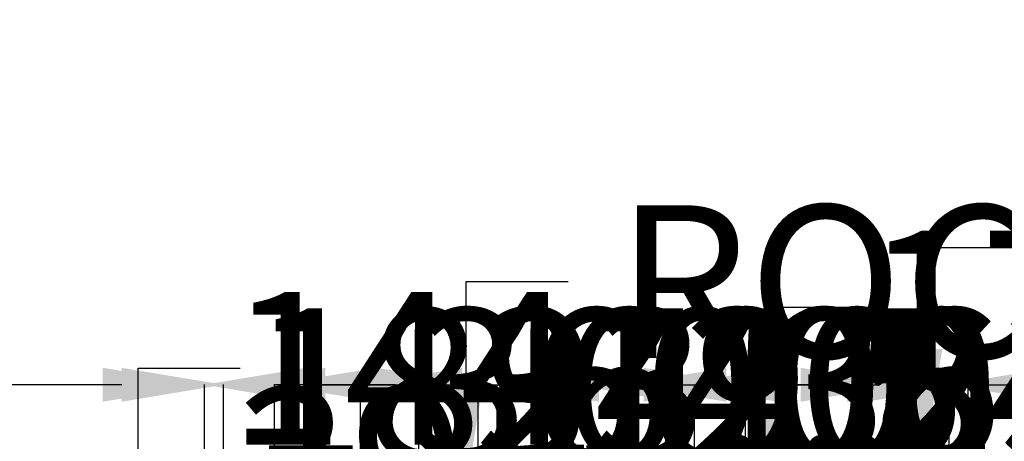
# Model space of a CAD drawing. Units: inches. Extents: x -307 to 2141, y -58 to 895.
# Tile 25 of 28: x 469 to 933, y 696 to 895. Entities that reach past the tile are written whole.
import ezdxf

# ---------------------------------------------------------------- set-up
doc = ezdxf.new("R2010")
doc.units = ezdxf.units.IN
doc.header["$MEASUREMENT"] = 0
doc.layers.add('A-ANNO-DIMS', color=2, linetype='Continuous', lineweight=18)
doc.styles.get("Standard").update_dxf_attribs({"font": 'arial.ttf'})
doc.dimstyles.get("Standard").update_dxf_attribs({"dimtxt": 72, "dimasz": 48, "dimexe": 0.18, "dimexo": 0.0625, "dimgap": 0.09, "dimtad": 0, "dimtih": 1, "dimtoh": 1, "dimdec": 0, "dimrnd": 48, "dimzin": 0, "dimdsep": 46, "dimlunit": 3, "dimtxsty": 'Standard', "dimcen": 0.09, "dimadec": 0, "dimazin": 0, "dimtfac": 1, "dimtdec": 0, "dimtofl": 0, "dimtmove": 0, "dimatfit": 3, "dimfxl": 1, "dimtolj": 1, "dimtzin": 0, "dimarcsym": 0})

# ---------------------------------------------------------------- blocks, each defined once
blk = doc.blocks.new('*D26')
at = {"layer": 'A-ANNO-DIMS', "color": 0, "lineweight": -2, "transparency": 16777216}
for p, q in [((565.34, 584.2), (565.34, 572.08)), ((645.34, 584.2), (645.34, 572.08)), ((517.34, 572.26), (469.34, 572.26)), ((693.34, 572.26), (741.34, 572.26))]:
    blk.add_line(p, q, dxfattribs=at)
at = {"layer": 'A-ANNO-DIMS', "color": 0, "transparency": 16777216}
for points in [[(517.34, 580.26), (517.34, 564.26), (565.34, 572.26)], [(693.34, 580.26), (693.34, 564.26), (645.34, 572.26)]]:
    blk.add_solid(points, dxfattribs=at)
at = {"layer": 'Defpoints', "color": 0, "transparency": 16777216}
for p in [(565.34, 584.26), (645.34, 584.26), (565.34, 572.26)]:
    blk.add_point(p, dxfattribs=at)
at = {"layer": 'A-ANNO-DIMS', "color": 0, "transparency": 16777216, "insert": (178.23, 572.26), "char_height": 72, "attachment_point": 5}
blk.add_mtext('\\A1;BED 80 TYP.', dxfattribs=at)
blk = doc.blocks.new('*D27')
at = {"layer": 'A-ANNO-DIMS', "color": 0, "lineweight": -2, "transparency": 16777216}
for p, q in [((657.34, 692.26), (657.34, 740.26)), ((645.4, 644.26), (657.52, 644.26)), ((645.4, 584.26), (657.52, 584.26)), ((657.34, 536.26), (657.34, 488.26)), ((657.34, 488.26), (609.34, 488.26))]:
    blk.add_line(p, q, dxfattribs=at)
at = {"layer": 'A-ANNO-DIMS', "color": 0, "transparency": 16777216}
for points in [[(649.34, 692.26), (665.34, 692.26), (657.34, 644.26)], [(649.34, 536.26), (665.34, 536.26), (657.34, 584.26)]]:
    blk.add_solid(points, dxfattribs=at)
at = {"layer": 'Defpoints', "color": 0, "transparency": 16777216}
for p in [(645.34, 644.26), (645.34, 584.26), (657.34, 584.26)]:
    blk.add_point(p, dxfattribs=at)
at = {"layer": 'A-ANNO-DIMS', "color": 0, "transparency": 16777216, "insert": (433.81, 488.26), "char_height": 72, "attachment_point": 5}
blk.add_mtext('\\A1;60 TYP.', dxfattribs=at)
blk = doc.blocks.new('*D30')
at = {"layer": 'A-ANNO-DIMS', "color": 0, "lineweight": -2, "transparency": 16777216}
for p, q in [((570.74, 532.83), (570.74, 580.83)), ((570.74, 580.83), (618.74, 580.83)), ((565.4, 484.83), (570.92, 484.83)), ((565.4, 448.83), (570.92, 448.83)), ((570.74, 400.83), (570.74, 352.83))]:
    blk.add_line(p, q, dxfattribs=at)
at = {"layer": 'A-ANNO-DIMS', "color": 0, "transparency": 16777216}
for points in [[(562.74, 532.83), (578.74, 532.83), (570.74, 484.83)], [(562.74, 400.83), (578.74, 400.83), (570.74, 448.83)]]:
    blk.add_solid(points, dxfattribs=at)
at = {"layer": 'Defpoints', "color": 0, "transparency": 16777216}
for p in [(565.34, 484.83), (570.74, 484.83), (565.34, 448.83)]:
    blk.add_point(p, dxfattribs=at)
at = {"layer": 'A-ANNO-DIMS', "color": 0, "transparency": 16777216, "insert": (1030.17, 580.83), "char_height": 72, "attachment_point": 5}
blk.add_mtext('\\A1;WINDOW 36 TYP.', dxfattribs=at)
blk = doc.blocks.new('*D32')
at = {"layer": 'A-ANNO-DIMS', "color": 0, "lineweight": -2, "transparency": 16777216}
for p, q in [((813.29, 682.28), (813.29, 671.36)), ((885.29, 682.28), (885.29, 671.36)), ((765.29, 671.54), (717.29, 671.54)), ((933.29, 671.54), (981.29, 671.54))]:
    blk.add_line(p, q, dxfattribs=at)
at = {"layer": 'A-ANNO-DIMS', "color": 0, "transparency": 16777216}
for points in [[(765.29, 679.54), (765.29, 663.54), (813.29, 671.54)], [(933.29, 679.54), (933.29, 663.54), (885.29, 671.54)]]:
    blk.add_solid(points, dxfattribs=at)
at = {"layer": 'Defpoints', "color": 0, "transparency": 16777216}
for p in [(813.29, 682.34), (885.29, 682.34), (885.29, 671.54)]:
    blk.add_point(p, dxfattribs=at)
at = {"layer": 'A-ANNO-DIMS', "color": 0, "transparency": 16777216, "insert": (1392.73, 671.54), "char_height": 72, "attachment_point": 5}
blk.add_mtext('\\A1;WINDOW 72 TYP.', dxfattribs=at)
blk = doc.blocks.new('*D33')
at = {"layer": 'A-ANNO-DIMS', "color": 0, "lineweight": -2, "transparency": 16777216}
for p, q in [((896.09, 739.34), (896.09, 787.34)), ((896.09, 787.34), (944.09, 787.34)), ((885.36, 691.34), (896.27, 691.34)), ((885.36, 682.34), (896.27, 682.34)), ((896.09, 634.34), (896.09, 586.34))]:
    blk.add_line(p, q, dxfattribs=at)
at = {"layer": 'A-ANNO-DIMS', "color": 0, "transparency": 16777216}
for points in [[(888.09, 739.34), (904.09, 739.34), (896.09, 691.34)], [(888.09, 634.34), (904.09, 634.34), (896.09, 682.34)]]:
    blk.add_solid(points, dxfattribs=at)
at = {"layer": 'Defpoints', "color": 0, "transparency": 16777216}
for p in [(885.29, 691.34), (896.09, 691.34), (885.29, 682.34)]:
    blk.add_point(p, dxfattribs=at)
at = {"layer": 'A-ANNO-DIMS', "color": 0, "transparency": 16777216, "insert": (1091.45, 787.34), "char_height": 72, "attachment_point": 5}
blk.add_mtext('\\A1;9 TYP.', dxfattribs=at)
blk = doc.blocks.new('*D34')
at = {"layer": 'A-ANNO-DIMS', "color": 0, "lineweight": -2, "transparency": 16777216}
for p, q in [((927.14, 490.97), (927.14, 538.97)), ((927.14, 538.97), (975.14, 538.97)), ((916.4, 442.97), (927.32, 442.97)), ((916.4, 370.95), (927.32, 370.95)), ((927.14, 322.95), (927.14, 274.95))]:
    blk.add_line(p, q, dxfattribs=at)
at = {"layer": 'A-ANNO-DIMS', "color": 0, "transparency": 16777216}
for points in [[(919.14, 490.97), (935.14, 490.97), (927.14, 442.97)], [(919.14, 322.95), (935.14, 322.95), (927.14, 370.95)]]:
    blk.add_solid(points, dxfattribs=at)
at = {"layer": 'Defpoints', "color": 0, "transparency": 16777216}
for p in [(916.34, 442.97), (927.14, 442.97), (916.34, 370.95)]:
    blk.add_point(p, dxfattribs=at)
at = {"layer": 'A-ANNO-DIMS', "color": 0, "transparency": 16777216, "insert": (1584.53, 538.97), "char_height": 72, "attachment_point": 5}
blk.add_mtext('\\A1;PAIRED WINDOW 72 TYP.', dxfattribs=at)
blk = doc.blocks.new('*D46')
at = {"layer": 'A-ANNO-DIMS', "color": 0, "lineweight": -2, "transparency": 16777216}
for p, q in [((801.41, 645.78), (801.41, 642.52)), ((822.41, 645.78), (822.41, 642.52)), ((753.41, 642.7), (705.41, 642.7)), ((870.41, 642.7), (918.41, 642.7))]:
    blk.add_line(p, q, dxfattribs=at)
at = {"layer": 'A-ANNO-DIMS', "color": 0, "transparency": 16777216}
for points in [[(753.41, 650.7), (753.41, 634.7), (801.41, 642.7)], [(870.41, 650.7), (870.41, 634.7), (822.41, 642.7)]]:
    blk.add_solid(points, dxfattribs=at)
at = {"layer": 'Defpoints', "color": 0, "transparency": 16777216}
for p in [(801.41, 645.85), (822.41, 645.85), (822.41, 642.7)]:
    blk.add_point(p, dxfattribs=at)
at = {"layer": 'A-ANNO-DIMS', "color": 0, "transparency": 16777216, "insert": (1282.7, 642.7), "char_height": 72, "attachment_point": 5}
blk.add_mtext('\\A1;DESK CHAIR 21', dxfattribs=at)
blk = doc.blocks.new('*D47')
at = {"layer": 'A-ANNO-DIMS', "color": 0, "lineweight": -2, "transparency": 16777216}
for p, q in [((825.56, 711.18), (825.56, 759.18)), ((825.56, 759.18), (873.56, 759.18)), ((822.48, 663.18), (825.74, 663.18)), ((822.48, 645.85), (825.74, 645.85)), ((825.56, 597.85), (825.56, 549.85))]:
    blk.add_line(p, q, dxfattribs=at)
at = {"layer": 'A-ANNO-DIMS', "color": 0, "transparency": 16777216}
for points in [[(817.56, 711.18), (833.56, 711.18), (825.56, 663.18)], [(817.56, 597.85), (833.56, 597.85), (825.56, 645.85)]]:
    blk.add_solid(points, dxfattribs=at)
at = {"layer": 'Defpoints', "color": 0, "transparency": 16777216}
for p in [(822.41, 663.18), (825.56, 663.18), (822.41, 645.85)]:
    blk.add_point(p, dxfattribs=at)
at = {"layer": 'A-ANNO-DIMS', "color": 0, "transparency": 16777216, "insert": (921.83, 759.18), "char_height": 72, "attachment_point": 5}
blk.add_mtext('\\A1;17', dxfattribs=at)
blk = doc.blocks.new('*D56')
at = {"layer": 'A-ANNO-DIMS', "color": 0, "lineweight": -2, "transparency": 16777216}
for p, q in [((679.73, 723.21), (679.73, 771.21)), ((679.73, 771.21), (727.73, 771.21)), ((675.74, 675.21), (679.91, 675.21)), ((675.74, 648.21), (679.91, 648.21)), ((679.73, 600.21), (679.73, 552.21))]:
    blk.add_line(p, q, dxfattribs=at)
at = {"layer": 'A-ANNO-DIMS', "color": 0, "transparency": 16777216}
for points in [[(671.73, 723.21), (687.73, 723.21), (679.73, 675.21)], [(671.73, 600.21), (687.73, 600.21), (679.73, 648.21)]]:
    blk.add_solid(points, dxfattribs=at)
at = {"layer": 'Defpoints', "color": 0, "transparency": 16777216}
for p in [(675.68, 675.21), (679.73, 675.21), (675.68, 648.21)]:
    blk.add_point(p, dxfattribs=at)
at = {"layer": 'A-ANNO-DIMS', "color": 0, "transparency": 16777216, "insert": (1006.66, 771.21), "char_height": 72, "attachment_point": 5}
blk.add_mtext('\\A1;ROCKER 27', dxfattribs=at)
blk = doc.blocks.new('*D62')
at = {"layer": 'A-ANNO-DIMS', "color": 0, "lineweight": -2, "transparency": 16777216}
for p, q in [((556.34, 691.4), (556.34, 722.72)), ((604.34, 722.54), (656.85, 722.54)), ((868.34, 722.54), (815.82, 722.54)), ((916.34, 490.97), (916.34, 722.72))]:
    blk.add_line(p, q, dxfattribs=at)
at = {"layer": 'A-ANNO-DIMS', "color": 0, "transparency": 16777216}
for points in [[(604.34, 730.54), (604.34, 714.54), (556.34, 722.54)], [(868.34, 730.54), (868.34, 714.54), (916.34, 722.54)]]:
    blk.add_solid(points, dxfattribs=at)
at = {"layer": 'Defpoints', "color": 0, "transparency": 16777216}
for p in [(916.34, 722.54), (556.34, 691.34), (916.34, 490.9)]:
    blk.add_point(p, dxfattribs=at)
at = {"layer": 'A-ANNO-DIMS', "color": 0, "transparency": 16777216, "insert": (736.34, 722.54), "char_height": 72, "attachment_point": 5}
blk.add_mtext('\\A1;360', dxfattribs=at)
blk = doc.blocks.new('*D69')
at = {"layer": 'A-ANNO-DIMS', "color": 0, "lineweight": -2, "transparency": 16777216}
for p, q in [((525.13, 682.34), (525.13, 730.34)), ((525.13, 730.34), (573.13, 730.34)), ((565.27, 682.34), (524.95, 682.34)), ((525.13, 586.34), (525.13, 634.34)), ((565.27, 538.34), (524.95, 538.34))]:
    blk.add_line(p, q, dxfattribs=at)
at = {"layer": 'A-ANNO-DIMS', "color": 0, "transparency": 16777216}
for points in [[(517.13, 634.34), (533.13, 634.34), (525.13, 682.34)], [(517.13, 586.34), (533.13, 586.34), (525.13, 538.34)]]:
    blk.add_solid(points, dxfattribs=at)
at = {"layer": 'Defpoints', "color": 0, "transparency": 16777216}
for p in [(525.13, 682.34), (565.34, 682.34), (565.34, 538.34)]:
    blk.add_point(p, dxfattribs=at)
at = {"layer": 'A-ANNO-DIMS', "color": 0, "transparency": 16777216, "insert": (649.22, 730.34), "char_height": 72, "attachment_point": 5}
blk.add_mtext('\\A1;144', dxfattribs=at)
blk = doc.blocks.new('*D75')
at = {"layer": 'A-ANNO-DIMS', "color": 0, "lineweight": -2, "transparency": 16777216}
for p, q in [((565.34, 682.4), (565.34, 722.72)), ((613.34, 722.54), (637.34, 722.54)), ((685.34, 682.4), (685.34, 722.72)), ((685.34, 722.54), (733.34, 722.54))]:
    blk.add_line(p, q, dxfattribs=at)
at = {"layer": 'A-ANNO-DIMS', "color": 0, "transparency": 16777216}
for points in [[(613.34, 730.54), (613.34, 714.54), (565.34, 722.54)], [(637.34, 730.54), (637.34, 714.54), (685.34, 722.54)]]:
    blk.add_solid(points, dxfattribs=at)
at = {"layer": 'Defpoints', "color": 0, "transparency": 16777216}
for p in [(685.34, 722.54), (565.34, 682.34), (685.34, 682.34)]:
    blk.add_point(p, dxfattribs=at)
at = {"layer": 'A-ANNO-DIMS', "color": 0, "transparency": 16777216, "insert": (809.45, 722.54), "char_height": 72, "attachment_point": 5}
blk.add_mtext('\\A1;120', dxfattribs=at)
blk = doc.blocks.new('*D76')
at = {"layer": 'A-ANNO-DIMS', "color": 0, "lineweight": -2, "transparency": 16777216}
for p, q in [((646.34, 722.54), (598.34, 722.54)), ((694.34, 682.4), (694.34, 722.72)), ((778.34, 682.4), (778.34, 722.72)), ((826.34, 722.54), (874.34, 722.54))]:
    blk.add_line(p, q, dxfattribs=at)
at = {"layer": 'A-ANNO-DIMS', "color": 0, "transparency": 16777216}
for points in [[(646.34, 730.54), (646.34, 714.54), (694.34, 722.54)], [(826.34, 730.54), (826.34, 714.54), (778.34, 722.54)]]:
    blk.add_solid(points, dxfattribs=at)
at = {"layer": 'Defpoints', "color": 0, "transparency": 16777216}
for p in [(778.34, 722.54), (694.34, 682.34), (778.34, 682.34)]:
    blk.add_point(p, dxfattribs=at)
at = {"layer": 'A-ANNO-DIMS', "color": 0, "transparency": 16777216, "insert": (925.9, 722.54), "char_height": 72, "attachment_point": 5}
blk.add_mtext('\\A1;84', dxfattribs=at)
blk = doc.blocks.new('*D77')
at = {"layer": 'A-ANNO-DIMS', "color": 0, "lineweight": -2, "transparency": 16777216}
for p, q in [((787.34, 682.4), (787.34, 722.72)), ((835.34, 722.54), (859.34, 722.54)), ((907.34, 682.4), (907.34, 722.72)), ((907.34, 722.54), (955.34, 722.54))]:
    blk.add_line(p, q, dxfattribs=at)
at = {"layer": 'A-ANNO-DIMS', "color": 0, "transparency": 16777216}
for points in [[(835.34, 730.54), (835.34, 714.54), (787.34, 722.54)], [(859.34, 730.54), (859.34, 714.54), (907.34, 722.54)]]:
    blk.add_solid(points, dxfattribs=at)
at = {"layer": 'Defpoints', "color": 0, "transparency": 16777216}
for p in [(907.34, 722.54), (787.34, 682.34), (907.34, 682.34)]:
    blk.add_point(p, dxfattribs=at)
at = {"layer": 'A-ANNO-DIMS', "color": 0, "transparency": 16777216, "insert": (1031.45, 722.54), "char_height": 72, "attachment_point": 5}
blk.add_mtext('\\A1;120', dxfattribs=at)
blk = doc.blocks.new('*D78')
at = {"layer": 'A-ANNO-DIMS', "color": 0, "lineweight": -2, "transparency": 16777216}
for p, q in [((947.53984, 730.340828), (947.53984, 778.340828)), ((778.39834, 682.340828), (947.71984, 682.340828)), ((730.39834, 598.340828), (947.71984, 598.340828)), ((947.53984, 550.340828), (947.53984, 502.340828))]:
    blk.add_line(p, q, dxfattribs=at)
at = {"layer": 'A-ANNO-DIMS', "color": 0, "transparency": 16777216}
for points in [[(939.53984, 730.340828), (955.53984, 730.340828), (947.53984, 682.340828)], [(939.53984, 550.340828), (955.53984, 550.340828), (947.53984, 598.340828)]]:
    blk.add_solid(points, dxfattribs=at)
at = {"layer": 'Defpoints', "color": 0, "transparency": 16777216}
for p in [(778.33584, 682.340828), (947.53984, 682.340828), (730.33584, 598.340828)]:
    blk.add_point(p, dxfattribs=at)
at = {"layer": 'A-ANNO-DIMS', "color": 0, "transparency": 16777216, "insert": (947.53984, 640.340828), "char_height": 72, "attachment_point": 5}
blk.add_mtext('\\A1;84', dxfattribs=at)
blk = doc.blocks.new('*D79')
at = {"layer": 'A-ANNO-DIMS', "color": 0, "lineweight": -2, "transparency": 16777216}
for p, q in [((947.54, 682.34), (947.54, 730.34)), ((947.54, 730.34), (995.54, 730.34)), ((907.4, 682.34), (947.72, 682.34)), ((947.54, 598.34), (947.54, 634.34)), ((907.4, 550.34), (947.72, 550.34))]:
    blk.add_line(p, q, dxfattribs=at)
at = {"layer": 'A-ANNO-DIMS', "color": 0, "transparency": 16777216}
for points in [[(939.54, 634.34), (955.54, 634.34), (947.54, 682.34)], [(939.54, 598.34), (955.54, 598.34), (947.54, 550.34)]]:
    blk.add_solid(points, dxfattribs=at)
at = {"layer": 'Defpoints', "color": 0, "transparency": 16777216}
for p in [(907.34, 682.34), (947.54, 682.34), (907.34, 550.34)]:
    blk.add_point(p, dxfattribs=at)
at = {"layer": 'A-ANNO-DIMS', "color": 0, "transparency": 16777216, "insert": (1071.41, 730.34), "char_height": 72, "attachment_point": 5}
blk.add_mtext('\\A1;132', dxfattribs=at)
blk = doc.blocks.new('*D80')
at = {"layer": 'A-ANNO-DIMS', "color": 0, "lineweight": -2, "transparency": 16777216}
for p, q in [((763.34, 722.54), (715.34, 722.54)), ((811.34, 517.4), (811.34, 722.72)), ((907.34, 541.4), (907.34, 722.72)), ((955.34, 722.54), (1003.34, 722.54))]:
    blk.add_line(p, q, dxfattribs=at)
at = {"layer": 'A-ANNO-DIMS', "color": 0, "transparency": 16777216}
for points in [[(763.34, 730.54), (763.34, 714.54), (811.34, 722.54)], [(955.34, 730.54), (955.34, 714.54), (907.34, 722.54)]]:
    blk.add_solid(points, dxfattribs=at)
at = {"layer": 'Defpoints', "color": 0, "transparency": 16777216}
for p in [(907.34, 722.54), (907.34, 541.34), (811.34, 517.34)]:
    blk.add_point(p, dxfattribs=at)
at = {"layer": 'A-ANNO-DIMS', "color": 0, "transparency": 16777216, "insert": (1054.97, 722.54), "char_height": 72, "attachment_point": 5}
blk.add_mtext('\\A1;96', dxfattribs=at)
blk = doc.blocks.new('*D88')
at = {"layer": 'A-ANNO-DIMS', "color": 0, "lineweight": -2, "transparency": 16777216}
for p, q in [((517.33584, 722.544828), (469.33584, 722.544828)), ((565.33584, 295.403328), (565.33584, 722.724828)), ((754.33584, 271.403328), (754.33584, 722.724828)), ((802.33584, 722.544828), (850.33584, 722.544828))]:
    blk.add_line(p, q, dxfattribs=at)
at = {"layer": 'A-ANNO-DIMS', "color": 0, "transparency": 16777216}
for points in [[(517.33584, 730.544828), (517.33584, 714.544828), (565.33584, 722.544828)], [(802.33584, 730.544828), (802.33584, 714.544828), (754.33584, 722.544828)]]:
    blk.add_solid(points, dxfattribs=at)
at = {"layer": 'Defpoints', "color": 0, "transparency": 16777216}
for p in [(754.33584, 722.544828), (565.33584, 295.340828), (754.33584, 271.340828)]:
    blk.add_point(p, dxfattribs=at)
at = {"layer": 'A-ANNO-DIMS', "color": 0, "transparency": 16777216, "insert": (659.83584, 722.544828), "char_height": 72, "attachment_point": 5}
blk.add_mtext('\\A1;189', dxfattribs=at)
blk = doc.blocks.new('*D94')
at = {"layer": 'A-ANNO-DIMS', "color": 0, "lineweight": -2, "transparency": 16777216}
for p, q in [((517.34, 722.54), (469.34, 722.54)), ((565.34, 529.4), (565.34, 722.72)), ((629.84, 529.4), (629.84, 722.72)), ((677.84, 722.54), (725.84, 722.54))]:
    blk.add_line(p, q, dxfattribs=at)
at = {"layer": 'A-ANNO-DIMS', "color": 0, "transparency": 16777216}
for points in [[(517.34, 730.54), (517.34, 714.54), (565.34, 722.54)], [(677.84, 730.54), (677.84, 714.54), (629.84, 722.54)]]:
    blk.add_solid(points, dxfattribs=at)
at = {"layer": 'Defpoints', "color": 0, "transparency": 16777216}
for p in [(629.84, 722.54), (565.34, 529.34), (629.84, 529.34)]:
    blk.add_point(p, dxfattribs=at)
at = {"layer": 'A-ANNO-DIMS', "color": 0, "transparency": 16777216, "insert": (819.9, 722.54), "char_height": 72, "attachment_point": 5}
blk.add_mtext('\\A1;64.5', dxfattribs=at)
blk = doc.blocks.new('*D96')
at = {"layer": 'A-ANNO-DIMS', "color": 0, "lineweight": -2, "transparency": 16777216}
for p, q in [((646.34, 722.54), (598.34, 722.54)), ((694.34, 598.4), (694.34, 722.72)), ((730.34, 598.4), (730.34, 722.72)), ((778.34, 722.54), (826.34, 722.54))]:
    blk.add_line(p, q, dxfattribs=at)
at = {"layer": 'A-ANNO-DIMS', "color": 0, "transparency": 16777216}
for points in [[(646.34, 730.54), (646.34, 714.54), (694.34, 722.54)], [(778.34, 730.54), (778.34, 714.54), (730.34, 722.54)]]:
    blk.add_solid(points, dxfattribs=at)
at = {"layer": 'Defpoints', "color": 0, "transparency": 16777216}
for p in [(730.34, 722.54), (694.34, 598.34), (730.34, 598.34)]:
    blk.add_point(p, dxfattribs=at)
at = {"layer": 'A-ANNO-DIMS', "color": 0, "transparency": 16777216, "insert": (877.95, 722.54), "char_height": 72, "attachment_point": 5}
blk.add_mtext('\\A1;36', dxfattribs=at)
blk = doc.blocks.new('*D97')
at = {"layer": 'A-ANNO-DIMS', "color": 0, "lineweight": -2, "transparency": 16777216}
for p, q in [((947.54, 637.34), (947.54, 685.34)), ((947.54, 685.34), (995.54, 685.34)), ((685.4, 589.34), (947.72, 589.34)), ((685.4, 538.34), (947.72, 538.34)), ((947.54, 490.34), (947.54, 442.34))]:
    blk.add_line(p, q, dxfattribs=at)
at = {"layer": 'A-ANNO-DIMS', "color": 0, "transparency": 16777216}
for points in [[(939.54, 637.34), (955.54, 637.34), (947.54, 589.34)], [(939.54, 490.34), (955.54, 490.34), (947.54, 538.34)]]:
    blk.add_solid(points, dxfattribs=at)
at = {"layer": 'Defpoints', "color": 0, "transparency": 16777216}
for p in [(685.34, 589.34), (947.54, 589.34), (685.34, 538.34)]:
    blk.add_point(p, dxfattribs=at)
at = {"layer": 'A-ANNO-DIMS', "color": 0, "transparency": 16777216, "insert": (1040.25, 685.34), "char_height": 72, "attachment_point": 5}
blk.add_mtext('\\A1;51', dxfattribs=at)
blk = doc.blocks.new('*D98')
at = {"layer": 'A-ANNO-DIMS', "color": 0, "lineweight": -2, "transparency": 16777216}
for p, q in [((525.13, 637.34), (525.13, 685.34)), ((525.13, 685.34), (573.13, 685.34)), ((787.27, 589.34), (524.95, 589.34)), ((787.27, 550.34), (524.95, 550.34)), ((525.13, 502.34), (525.13, 454.34))]:
    blk.add_line(p, q, dxfattribs=at)
at = {"layer": 'A-ANNO-DIMS', "color": 0, "transparency": 16777216}
for points in [[(517.13, 637.34), (533.13, 637.34), (525.13, 589.34)], [(517.13, 502.34), (533.13, 502.34), (525.13, 550.34)]]:
    blk.add_solid(points, dxfattribs=at)
at = {"layer": 'Defpoints', "color": 0, "transparency": 16777216}
for p in [(525.13, 589.34), (787.34, 589.34), (787.34, 550.34)]:
    blk.add_point(p, dxfattribs=at)
at = {"layer": 'A-ANNO-DIMS', "color": 0, "transparency": 16777216, "insert": (624.84, 685.34), "char_height": 72, "attachment_point": 5}
blk.add_mtext('\\A1;39', dxfattribs=at)
blk = doc.blocks.new('*D101')
at = {"layer": 'A-ANNO-DIMS', "color": 0, "lineweight": -2, "transparency": 16777216}
for p, q in [((508.34, 722.54), (460.34, 722.54)), ((556.34, 691.4), (556.34, 722.72)), ((589.36, 691.4), (589.36, 722.72)), ((637.36, 722.54), (685.36, 722.54))]:
    blk.add_line(p, q, dxfattribs=at)
at = {"layer": 'A-ANNO-DIMS', "color": 0, "transparency": 16777216}
for points in [[(508.34, 730.54), (508.34, 714.54), (556.34, 722.54)], [(637.36, 730.54), (637.36, 714.54), (589.36, 722.54)]]:
    blk.add_solid(points, dxfattribs=at)
at = {"layer": 'Defpoints', "color": 0, "transparency": 16777216}
for p in [(589.36, 722.54), (556.34, 691.34), (589.36, 691.34)]:
    blk.add_point(p, dxfattribs=at)
at = {"layer": 'A-ANNO-DIMS', "color": 0, "transparency": 16777216, "insert": (806.54, 722.54), "char_height": 72, "attachment_point": 5}
blk.add_mtext('\\A1;33.02', dxfattribs=at)
blk = doc.blocks.new('*D102')
at = {"layer": 'A-ANNO-DIMS', "color": 0, "lineweight": -2, "transparency": 16777216}
for p, q in [((837.29, 722.54), (789.29, 722.54)), ((885.29, 691.4), (885.29, 722.72)), ((916.34, 691.4), (916.34, 722.72)), ((964.34, 722.54), (1012.34, 722.54))]:
    blk.add_line(p, q, dxfattribs=at)
at = {"layer": 'A-ANNO-DIMS', "color": 0, "transparency": 16777216}
for points in [[(837.29, 730.54), (837.29, 714.54), (885.29, 722.54)], [(964.34, 730.54), (964.34, 714.54), (916.34, 722.54)]]:
    blk.add_solid(points, dxfattribs=at)
at = {"layer": 'Defpoints', "color": 0, "transparency": 16777216}
for p in [(916.34, 722.54), (885.29, 691.34), (916.34, 691.34)]:
    blk.add_point(p, dxfattribs=at)
at = {"layer": 'A-ANNO-DIMS', "color": 0, "transparency": 16777216, "insert": (1133.74, 722.54), "char_height": 72, "attachment_point": 5}
blk.add_mtext('\\A1;31.04', dxfattribs=at)
blk = doc.blocks.new('*D103')
at = {"layer": 'A-ANNO-DIMS', "color": 0, "lineweight": -2, "transparency": 16777216}
for p, q in [((637.34, 722.54), (589.34, 722.54)), ((685.34, 682.4), (685.34, 722.72)), ((694.34, 682.4), (694.34, 722.72)), ((742.34, 722.54), (790.34, 722.54))]:
    blk.add_line(p, q, dxfattribs=at)
at = {"layer": 'A-ANNO-DIMS', "color": 0, "transparency": 16777216}
for points in [[(637.34, 730.54), (637.34, 714.54), (685.34, 722.54)], [(742.34, 730.54), (742.34, 714.54), (694.34, 722.54)]]:
    blk.add_solid(points, dxfattribs=at)
at = {"layer": 'Defpoints', "color": 0, "transparency": 16777216}
for p in [(694.34, 722.54), (685.34, 682.34), (694.34, 682.34)]:
    blk.add_point(p, dxfattribs=at)
at = {"layer": 'A-ANNO-DIMS', "color": 0, "transparency": 16777216, "insert": (814.1, 722.54), "char_height": 72, "attachment_point": 5}
blk.add_mtext('\\A1;9', dxfattribs=at)
blk = doc.blocks.new('*D107')
at = {"layer": 'A-ANNO-DIMS', "color": 0, "lineweight": -2, "transparency": 16777216}
for p, q in [((517.34, 722.54), (469.34, 722.54)), ((565.34, 409.4), (565.34, 722.72)), ((589.34, 409.4), (589.34, 722.72)), ((637.34, 722.54), (685.34, 722.54))]:
    blk.add_line(p, q, dxfattribs=at)
at = {"layer": 'A-ANNO-DIMS', "color": 0, "transparency": 16777216}
for points in [[(517.34, 730.54), (517.34, 714.54), (565.34, 722.54)], [(637.34, 730.54), (637.34, 714.54), (589.34, 722.54)]]:
    blk.add_solid(points, dxfattribs=at)
at = {"layer": 'Defpoints', "color": 0, "transparency": 16777216}
for p in [(589.34, 722.54), (565.34, 409.34), (589.34, 409.34)]:
    blk.add_point(p, dxfattribs=at)
at = {"layer": 'A-ANNO-DIMS', "color": 0, "transparency": 16777216, "insert": (835.49, 722.54), "char_height": 72, "attachment_point": 5}
blk.add_mtext('\\A1;24.003', dxfattribs=at)

msp = doc.modelspace()

# ---------------------------------------------------------------- dimensions: what is measured, and where the dimension line sits
at = {"layer": 'A-ANNO-DIMS'}
for base, p1, p2, angle, text, picture, middle in [((896.0934, 691.3408), (885.2934, 682.3408), (885.2934, 691.3408), 90, '<> TYP.', '*D33', (1091.4494, 787.3408)), ((679.7317, 675.211), (675.6817, 648.211), (675.6817, 675.211), 90, 'ROCKER <>', '*D56', (1006.6621, 771.211)), ((927.1381, 442.9669), (916.3358, 370.9517), (916.3358, 442.9669), 90, 'PAIRED WINDOW <> TYP.', '*D34', (1584.5269, 538.9669)), ((570.7358, 484.8333), (565.3358, 448.8333), (565.3358, 484.8333), 90, 'WINDOW <> TYP.', '*D30', (1030.1737, 580.8333)), ((565.3358, 572.2648), (645.3359, 584.2648), (565.3358, 584.2648), 180, 'BED <> TYP.', '*D26', (178.2254, 572.2648)), ((657.3359, 584.2648), (645.3359, 644.2648), (645.3359, 584.2648), 270, '<> TYP.', '*D27', (433.8134, 488.2648))]:
    dim = msp.add_linear_dim(base=base, p1=p1, p2=p2, angle=angle, text=text, dimstyle='Standard', override={"dimdec": 0, "dimlfac": 1, "dimrnd": 0, "dimzin": 0, "dimdsep": 46, "dimlunit": 2}, dxfattribs=at)
    dim.commit()
    dim.dimension.update_dxf_attribs({"geometry": picture, "text_midpoint": middle})
for base, p1, p2, text, picture, middle in [((885.2934, 671.5408), (813.2934, 682.3408), (885.2934, 682.3408), 'WINDOW <> TYP.', '*D32', (1392.7312, 671.5408)), ((822.4132, 642.696), (801.4132, 645.846), (822.4132, 645.846), 'DESK CHAIR <>', '*D46', (1282.7024, 642.696))]:
    dim = msp.add_linear_dim(base=base, p1=p1, p2=p2, text=text, dimstyle='Standard', override={"dimdec": 0, "dimlfac": 1, "dimrnd": 0, "dimzin": 0, "dimdsep": 46, "dimlunit": 2}, dxfattribs=at)
    dim.commit()
    dim.dimension.update_dxf_attribs({"geometry": picture, "text_midpoint": middle})
for base, p1, p2, picture, middle in [((825.5632, 663.1793), (822.4132, 645.846), (822.4132, 663.1793), '*D47', (921.8333, 759.1793)), ((525.1318, 682.3408), (565.3358, 538.3408), (565.3358, 682.3408), '*D69', (649.2246, 730.3408)), ((947.5398, 682.3408), (730.3358, 598.3408), (778.3358, 682.3408), '*D78', (947.5398, 640.3408)), ((947.5398, 682.3408), (907.3358, 550.3408), (907.3358, 682.3408), '*D79', (1071.4116, 730.3408)), ((525.1318, 589.3408), (787.3358, 550.3408), (787.3358, 589.3408), '*D98', (624.8398, 685.3408)), ((947.5398, 589.3408), (685.3358, 538.3408), (685.3358, 589.3408), '*D97', (1040.2492, 685.3408))]:
    dim = msp.add_linear_dim(base=base, p1=p1, p2=p2, angle=90, dimstyle='Standard', override={"dimdec": 0, "dimlfac": 1, "dimrnd": 0, "dimzin": 0, "dimdsep": 46, "dimlunit": 2}, dxfattribs=at)
    dim.commit()
    dim.dimension.update_dxf_attribs({"geometry": picture, "text_midpoint": middle})
for base, p1, p2, override, picture, middle in [((589.3579, 722.5448), (556.3358, 691.3408), (589.3579, 691.3408), {"dimdec": 2, "dimlfac": 1, "dimrnd": 0, "dimzin": 0, "dimdsep": 46, "dimlunit": 2}, '*D101', (806.5366, 722.5448)), ((754.3358, 722.5448), (565.3358, 295.3408), (754.3358, 271.3408), {"dimdec": 0, "dimlfac": 1, "dimrnd": 0, "dimzin": 0, "dimdsep": 46, "dimlunit": 2}, '*D88', (659.8358, 722.5448)), ((629.8358, 722.5448), (565.3358, 529.3408), (629.8358, 529.3408), {"dimdec": 1, "dimlfac": 1, "dimrnd": 0, "dimzin": 0, "dimdsep": 46, "dimlunit": 2}, '*D94', (819.904, 722.5448)), ((589.339, 722.5448), (565.3358, 409.3408), (589.339, 409.3408), {"dimdec": 3, "dimlfac": 1, "dimrnd": 0, "dimzin": 0, "dimdsep": 46, "dimlunit": 2}, '*D107', (835.4945, 722.5448)), ((916.3358, 722.5448), (556.3358, 691.3408), (916.3358, 490.9034), {"dimdec": 0, "dimlfac": 1, "dimrnd": 0, "dimzin": 0, "dimdsep": 46, "dimlunit": 2}, '*D62', (736.3358, 722.5448)), ((685.3358, 722.5448), (565.3358, 682.3408), (685.3358, 682.3408), {"dimdec": 0, "dimlfac": 1, "dimrnd": 0, "dimzin": 0, "dimdsep": 46, "dimlunit": 2}, '*D75', (809.4531, 722.5448)), ((694.3358, 722.5448), (685.3358, 682.3408), (694.3358, 682.3408), {"dimdec": 0, "dimlfac": 1, "dimrnd": 0, "dimzin": 0, "dimdsep": 46, "dimlunit": 2}, '*D103', (814.0984, 722.5448)), ((778.3358, 722.5448), (694.3358, 682.3408), (778.3358, 682.3408), {"dimdec": 0, "dimlfac": 1, "dimrnd": 0, "dimzin": 0, "dimdsep": 46, "dimlunit": 2}, '*D76', (925.8965, 722.5448)), ((730.3358, 722.5448), (694.3358, 598.3408), (730.3358, 598.3408), {"dimdec": 0, "dimlfac": 1, "dimrnd": 0, "dimzin": 0, "dimdsep": 46, "dimlunit": 2}, '*D96', (877.9456, 722.5448)), ((907.3358, 722.5448), (811.3358, 517.3408), (907.3358, 541.3408), {"dimdec": 0, "dimlfac": 1, "dimrnd": 0, "dimzin": 0, "dimdsep": 46, "dimlunit": 2}, '*D80', (1054.9702, 722.5448)), ((907.3358, 722.5448), (787.3358, 682.3408), (907.3358, 682.3408), {"dimdec": 0, "dimlfac": 1, "dimrnd": 0, "dimzin": 0, "dimdsep": 46, "dimlunit": 2}, '*D77', (1031.4531, 722.5448)), ((916.3358, 722.5448), (885.2934, 691.3408), (916.3358, 691.3408), {"dimdec": 2, "dimlfac": 1, "dimrnd": 0, "dimzin": 0, "dimdsep": 46, "dimlunit": 2}, '*D102', (1133.7355, 722.5448))]:
    dim = msp.add_linear_dim(base=base, p1=p1, p2=p2, dimstyle='Standard', override=override, dxfattribs=at)
    dim.commit()
    dim.dimension.update_dxf_attribs({"geometry": picture, "text_midpoint": middle})

doc.saveas('drawing.dxf')
